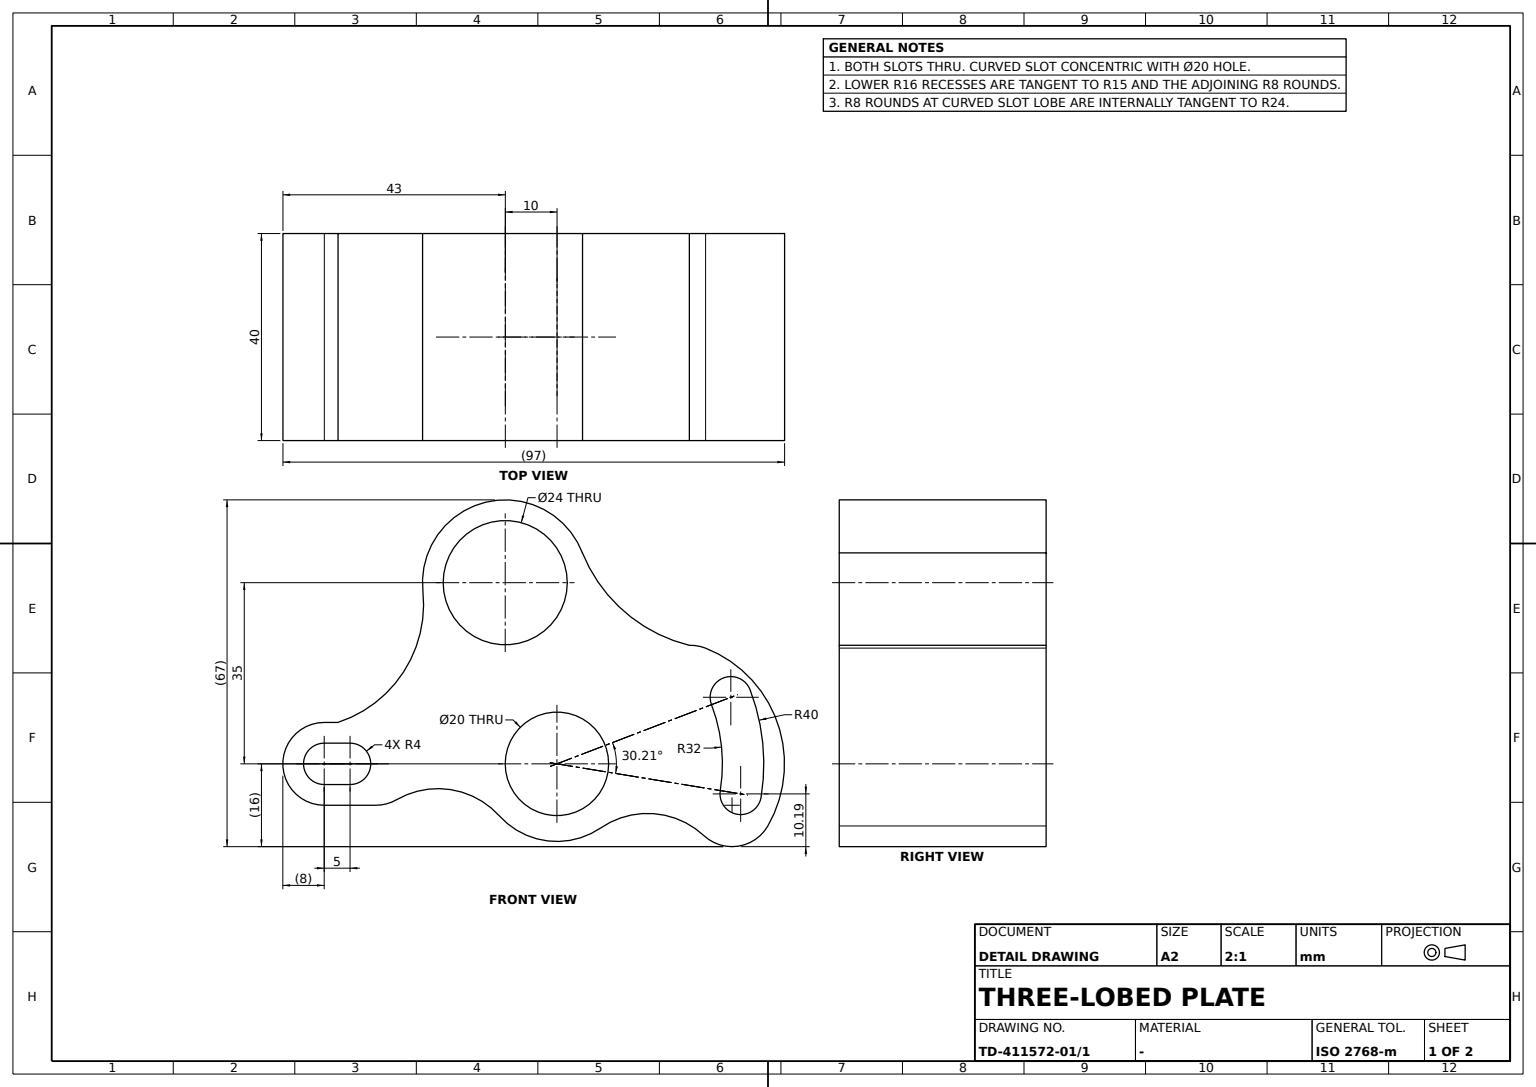
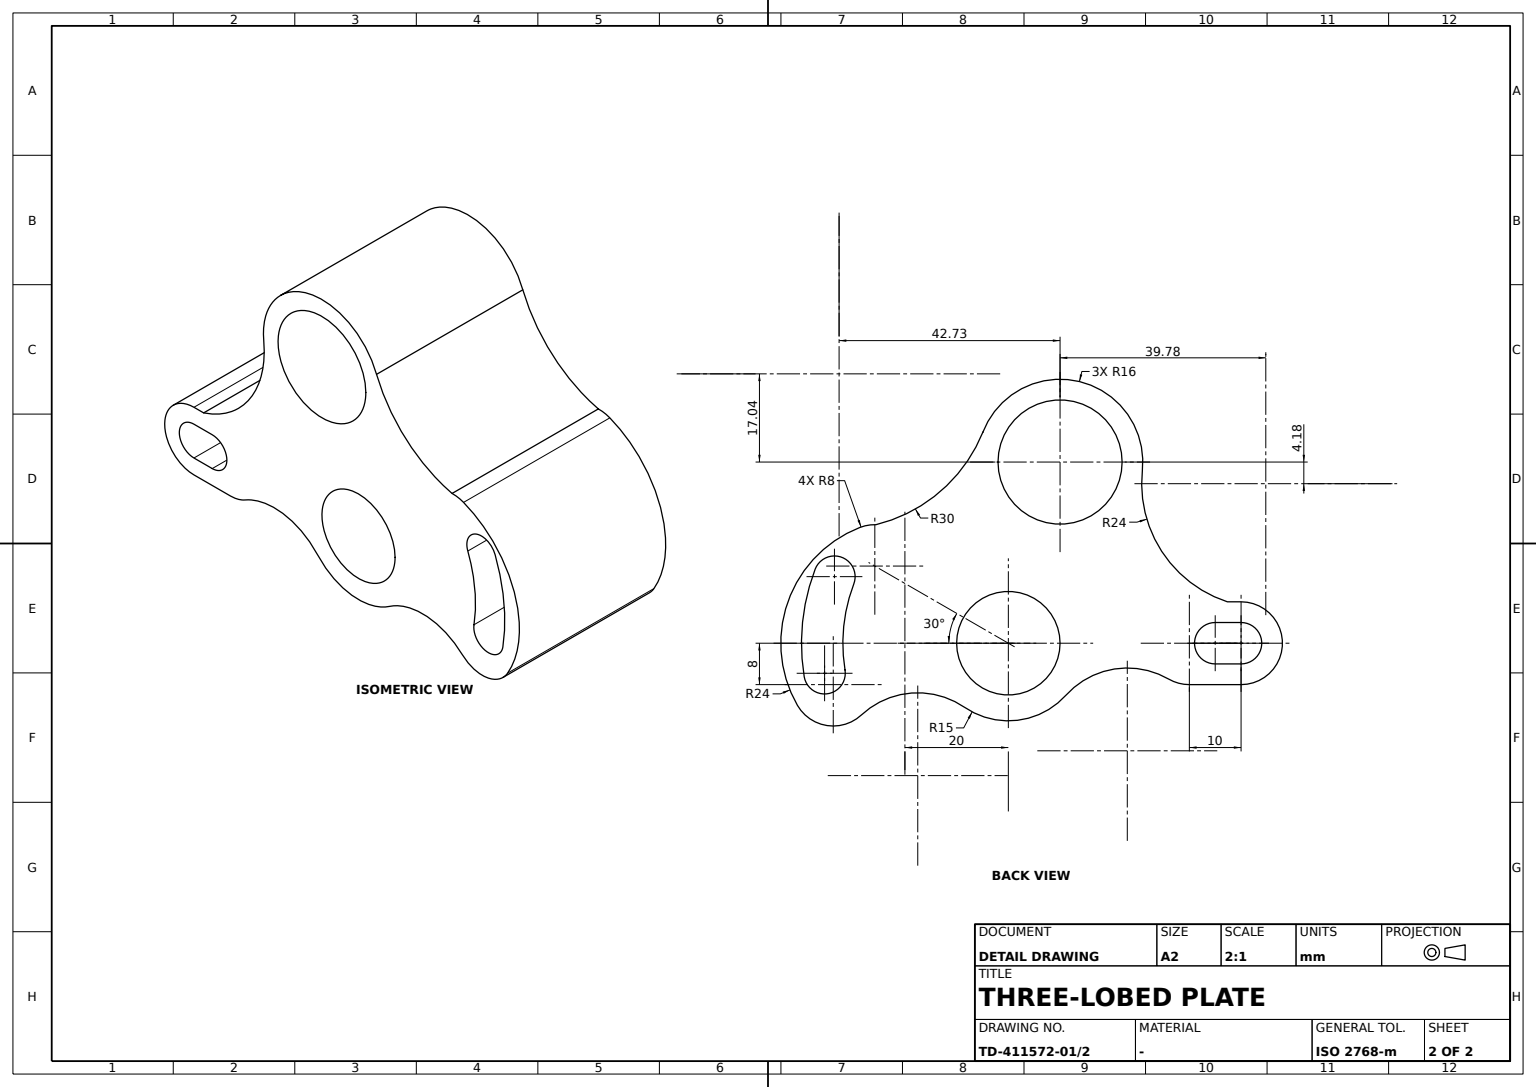
CATIA V5 part; units mm, degrees
sketch "Sketch1" plane through (0, 0, 0) normal (0, 0, 1) x (1, 0, 0)
  arc A0 (14.9285, 5.7566) -> (-15.9124, -1.6724) centre (0, 0) ccw
  point P0 (0, -12)
  point P1 (10, -35)
  arc A1 (-1.129, -45.0571) -> (18.4752, -47.3762) centre (10, -35) ccw
  line L0 (10, -35) -> (35.8167, -20.0947) construction
  arc A2 (43.8564, -43) -> (35.8167, -20.0947) centre (30, -35) ccw construction
  point P2 (30, -35)
  arc A3 (43.8564, -43) -> (35.8167, -20.0947) centre (30, -35) ccw construction
  arc A4 (50.7846, -47) -> (38.4094, -48.8592) centre (43.8564, -43) cw
  arc A5 (38.725, -12.6421) -> (50.7846, -47) centre (30, -35) cw
  arc A6 (14.9285, 5.7566) -> (35.5821, -12.0982) centre (42.7263, 17.0387) ccw
  arc A7 (18.4752, -47.3762) -> (38.4094, -48.8592) centre (27.5154, -60.5776) cw
  line L1 (-35, -35) -> (-25, -35) construction
  point P3 (-35, -35)
  line L2 (-35, -27) -> (-32.3452, -27)
  line L3 (-25, -43) -> (-35, -43)
  arc A8 (-21, -41.9282) -> (-25, -43) centre (-25, -35) cw
  arc A9 (-35, -43) -> (-35, -27) centre (-35, -35) cw
  line L4 (-35, -35) -> (-25, -35) construction
  arc A10 (-21, -41.9282) -> (-1.129, -45.0571) centre (-13, -55.7846) cw
  arc A11 (-15.9124, -1.6724) -> (-32.3452, -27) centre (-39.7809, -4.1809) cw
  arc A12 (35.5821, -12.0982) -> (38.725, -12.6421) centre (35.8167, -20.0947) cw
  dimension "radius A0" = 16
  dimension "radius A1" = 15
  dimension "distance P1 origin x axis" = 10
  dimension "distance P1 A3" = 36
  dimension "radius A6" = 30
  dimension "radius A7" = 16
  dimension "distance L1 L2" = 8
  dimension "radius A10" = 16
  dimension "radius A11" = 24
  dimension "length L4" = 10
  dimension "distance P3 A3" = 81
  constraint coincidence P0 y-axis
  constraint tangency A5 A4
  constraint tangency A7 A1
  constraint tangency A7 A4
  constraint tangency L1 A4
  constraint tangency A9 L2
  constraint tangency A8 L3
  constraint tangency A9 L3
  constraint tangency A10 A8
  constraint tangency A10 A1
  constraint tangency A11 A0
  constraint concentricity A5 P2
extrude "Pad1" add sketch "Sketch1" along normal mid plane 40
sketch "Sketch2" plane through (0, 0, 20) normal (0, 0, 1) x (1, 0, 0)
  circle A0 centre (0, 0) radius 12
  arc A1 (14.9285, 5.7566) -> (-15.9124, -1.6724) centre (0, 0) ccw construction
  circle A2 centre (10, -35) radius 10
  point P0 (10, -35)
  arc A3 (-1.129, -45.0571) -> (18.4752, -47.3762) centre (10, -35) ccw construction
  line L0 (-35, -35) -> (-30, -35) construction
  line L1 (-35, -31) -> (-30, -31)
  line L2 (-30, -39) -> (-35, -39)
  arc A4 (-30, -31) -> (-30, -39) centre (-30, -35) cw
  arc A5 (-35, -39) -> (-35, -31) centre (-35, -35) cw
  arc A6 (-35, -27) -> (-35, -43) centre (-35, -35) ccw construction
  arc A7 (50.7846, -47) -> (38.725, -12.6421) centre (30, -35) ccw construction
  line L3 (10, -35) -> (59.1976, -6.5957) construction
  line L4 (-60, -35) -> (80, -35) construction
  point P1 (-60, -35)
  arc A8 (45.5287, -40.8065) -> (43.6245, -22.1394) centre (10, -35) ccw construction
  arc A9 (49.4763, -41.4516) -> (41.581, -40.1613) centre (45.5287, -40.8065) cw
  arc A10 (39.8884, -23.5683) -> (47.3605, -20.7104) centre (43.6245, -22.1394) cw
  arc A11 (41.581, -40.1613) -> (39.8884, -23.5683) centre (10, -35) ccw
  arc A12 (47.3605, -20.7104) -> (49.4763, -41.4516) centre (10, -35) cw
  dimension "radius A0" = 12
  dimension "radius A2" = 10
  dimension "distance L0 L1" = 4
  dimension "radius A7" = 24
  dimension "angle L3 L4" = 30
  dimension "radius A10" = 4
  dimension "distance P0 A8" = 36
  constraint concentricity A0 A1
  constraint concentricity A2 A3
  constraint concentricity A6 A5
  constraint concentricity A11 P0
  constraint concentricity A12 P0
  constraint horizontal L0 x-axis
  constraint tangency A4 L1
  constraint tangency A5 L1
  constraint tangency A4 L2
  constraint tangency A5 L2
  constraint tangency A8 A4
  constraint tangency A11 A10
  constraint tangency A10 A12
  constraint tangency A12 A9
  constraint tangency A9 A11
  constraint coincidence P1 L0
extrude "Pocket1" cut sketch "Sketch2" against normal up to next
